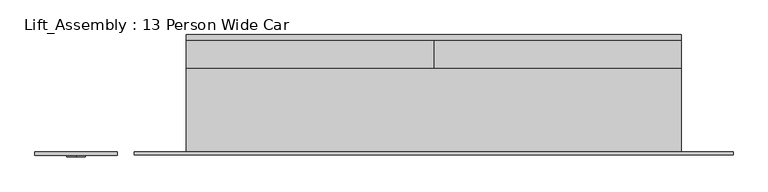
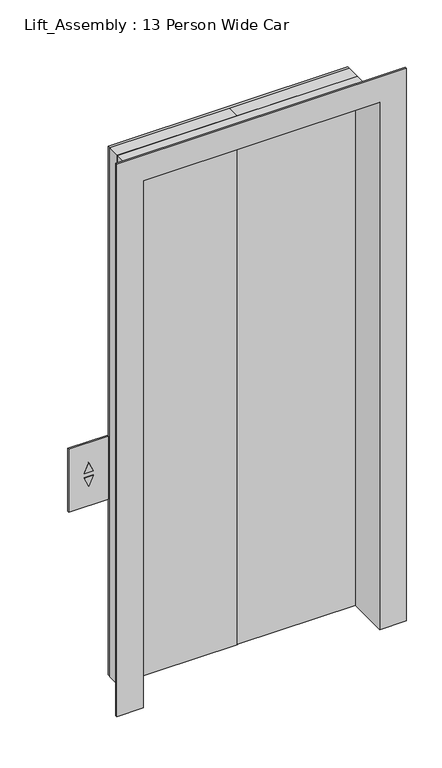
"""IFC4 building model written with IfcOpenShell, lengths in millimetres: proxy geometry, Lift_Assembly : 13 Person Wide Car."""

from ifc_helpers import new_model, si_unit, frame, origin, origin_with_axes, place, context, project, spatial, polyline, outline, extrude, faceted_brep, source, transform, mapped, element, save


def lift_assembly_13_person_wide_car_39bd1a5e(model_context):
    return source(origin(), model_context, "Body", "SolidModel", [
        extrude(outline(polyline([(200.0, 126.2), (200.0, 76.2), (-249.0, 76.2), (-249.0, 126.2), (200.0, 126.2)])), origin_with_axes(), (0.0, 0.0, 1.0), 2100.0),
        extrude(outline(polyline([(-250.0, 126.2), (-250.0, 76.2), (-700.0, 76.2), (-700.0, 126.2), (-250.0, 126.2)])), origin_with_axes(), (0.0, 0.0, 1.0), 2100.0),
        extrude(outline(polyline([(1008.7476885, -883.0952695), (1045.0, -900.0), (1008.7476885, -916.9047305), (1008.7476885, -883.0952695)])), frame((0.0, -85.2, 0.0), z_axis=(0.0, 1.0, 0.0), x_axis=(0.0, 0.0, 1.0)), (0.0, 0.0, 1.0), 9.0),
        extrude(outline(polyline([(991.2523115, -883.0952695), (991.2523115, -916.9047305), (955.0, -900.0), (991.2523115, -883.0952695)])), frame((0.0, -85.2, 0.0), z_axis=(0.0, 1.0, 0.0), x_axis=(0.0, 0.0, 1.0)), (0.0, 0.0, 1.0), 9.0),
        faceted_brep([(294.0, -82.2, 0.0), (194.0, -82.2, 0.0), (194.0, 136.8, 0.0), (200.0, 136.8, 0.0), (200.0, -76.2, 0.0), (294.0, -76.2, 0.0), (294.0, -76.2, 2194.0), (294.0, -82.2, 2194.0), (200.0, -76.2, 2100.0), (-700.0, -76.2, 2100.0), (-700.0, -76.2, 0.0), (-794.0, -76.2, 0.0), (-794.0, -76.2, 2194.0), (200.0, 136.8, 2100.0), (194.0, 136.8, 2094.0), (-694.0, 136.8, 2094.0), (-694.0, 136.8, 0.0), (-700.0, 136.8, 0.0), (-700.0, 136.8, 2100.0), (194.0, -82.2, 2094.0), (-794.0, -82.2, 2194.0), (-794.0, -82.2, 0.0), (-694.0, -82.2, 0.0), (-694.0, -82.2, 2094.0)], [[[0, 1, 2, 3, 4, 5]], [[5, 6, 7, 0]], [[4, 8, 9, 10, 11, 12, 6, 5]], [[3, 13, 8, 4]], [[2, 14, 15, 16, 17, 18, 13, 3]], [[1, 19, 14, 2]], [[0, 7, 20, 21, 22, 23, 19, 1]], [[6, 12, 20, 7]], [[13, 18, 9, 8]], [[19, 23, 15, 14]], [[21, 11, 10, 17, 16, 22]], [[12, 11, 21, 20]], [[18, 17, 10, 9]], [[23, 22, 16, 15]]]),
        extrude(outline(polyline([(875.0, -975.0), (875.0, -825.0), (1125.0, -825.0), (1125.0, -975.0), (875.0, -975.0)]), holes=[polyline([(1008.7476885, -883.0952695), (1008.7476885, -916.9047305), (1045.0, -900.0), (1008.7476885, -883.0952695)]), polyline([(991.2523115, -883.0952695), (955.0, -900.0), (991.2523115, -916.9047305), (991.2523115, -883.0952695)])]), frame((0.0, -82.2, 0.0), z_axis=(0.0, 1.0, 0.0), x_axis=(0.0, 0.0, 1.0)), (0.0, 0.0, 1.0), 6.0),
    ])


if __name__ == "__main__":
    model = new_model("IFC4")
    model_context = context("Model", 3, world=origin())
    ifc_project = project(units=[si_unit("LENGTHUNIT", "METRE", prefix="MILLI")], contexts=[model_context])
    site = spatial("IfcSite", under=ifc_project)
    building = spatial("IfcBuilding", under=site)
    placement = place(None, origin())
    lift_assembly_13_person_wide_car_shape = lift_assembly_13_person_wide_car_39bd1a5e(model_context)
    element("IfcBuildingElementProxy", 1, Name="Lift_Assembly : 13 Person Wide Car", ObjectType="Lift_Assembly : 13 Person Wide Car", at=placement, inside=building, context=model_context, shape_type="MappedRepresentation", body=[
        mapped(lift_assembly_13_person_wide_car_shape, transform((0.0, 0.0, 0.0), x_axis=(1.0, 0.0, 0.0), y_axis=(0.0, 1.0, 0.0), z_axis=(0.0, 0.0, 1.0))),
    ])
    save(model, "model.ifc")

# Revit data of these elements
# Type "Lift_Assembly : 13 Person Wide Car"
#   Keynote = "X"
#   Hoistway Width = 2400 mm
#   Hoistway Depth = 1800 mm
#   Height = 2100 mm
#   Frame Width = 75 mm
#   Percentage Opened (Plan) = 0 mm
#   Door Width = 900 mm
#   Door Trim Width = 100 mm
#   Door Thickness = 50 mm
#   Car Width = 1600 mm
#   Car Thickness = 25 mm
#   Car Front Offset = 250 mm
#   Car Depth = 1400 mm
#   Call Point Z Offset = 1000 mm
#   Call Point X Offset = 200 mm
#   Call Point Panel Width = 150 mm
#   Call Point Panel Depth = 250 mm
#   Vis - Hoistway Location Lines = yes
#   Vis - Door Trim = yes
#   Vis - Call Point = yes
#   Material Trim = Metal - Stainless Steel
#   Material Doors = Metal - Aluminium
#   Wall Closure = (empty or 0)
#   Default Elevation = 0
# Element 1 (IfcBuildingElementProxy, "Lift_Assembly : 13 Person Wide Car")
#   Materials on its faces: "Metal - Stainless Steel", "Metal - Aluminium"
# Materials
#   "Metal - Stainless Steel": class "Metal", colour RGB 247 247 247, transparency 0
#   "Metal - Aluminium": class "Metal", colour RGB 247 247 247, transparency 0
